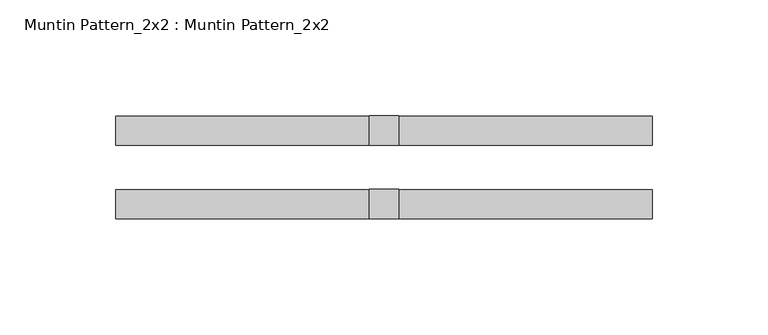
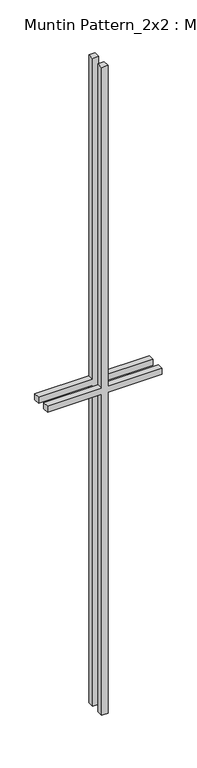
"""IFC4 building model written with IfcOpenShell, lengths in millimetres: proxy geometry, Muntin Pattern_2x2 : Muntin Pattern_2x2."""

from ifc_helpers import new_model, si_unit, frame, origin, place, context, project, spatial, polyline, outline, extrude, source, transform, mapped, element, save


def muntin_pattern_2x2_muntin_pattern_2x2_a2bda2b8(model_context):
    return source(origin(), model_context, "Body", "SweptSolid", [
        extrude(outline(polyline([(698.5, -6.35), (698.5, -115.8875), (685.8, -115.8875), (685.8, -6.35), (0.0, -6.35), (0.0, 6.35), (685.8, 6.35), (685.8, 115.8875), (698.5, 115.8875), (698.5, 6.35), (1384.3, 6.35), (1384.3, -6.35), (698.5, -6.35)])), frame((0.0, 9.525, 0.0), z_axis=(0.0, 1.0, 0.0), x_axis=(0.0, 0.0, 1.0)), (0.0, 0.0, 1.0), 12.7),
        extrude(outline(polyline([(698.5, -6.35), (698.5, -115.8875), (685.8, -115.8875), (685.8, -6.35), (0.0, -6.35), (0.0, 6.35), (685.8, 6.35), (685.8, 115.8875), (698.5, 115.8875), (698.5, 6.35), (1384.3, 6.35), (1384.3, -6.35), (698.5, -6.35)])), frame((0.0, -22.225, 0.0), z_axis=(0.0, 1.0, 0.0), x_axis=(0.0, 0.0, 1.0)), (0.0, 0.0, 1.0), 12.7),
    ])


if __name__ == "__main__":
    model = new_model("IFC4")
    model_context = context("Model", 3, world=origin())
    ifc_project = project(units=[si_unit("LENGTHUNIT", "METRE", prefix="MILLI")], contexts=[model_context])
    site = spatial("IfcSite", under=ifc_project)
    building = spatial("IfcBuilding", under=site)
    placement = place(None, origin())
    muntin_pattern_2x2_muntin_pattern_2x2_shape = muntin_pattern_2x2_muntin_pattern_2x2_a2bda2b8(model_context)
    element("IfcBuildingElementProxy", 1, Name="Muntin Pattern_2x2 : Muntin Pattern_2x2", ObjectType="Muntin Pattern_2x2 : Muntin Pattern_2x2", at=placement, inside=building, context=model_context, shape_type="MappedRepresentation", body=[
        mapped(muntin_pattern_2x2_muntin_pattern_2x2_shape, transform((0.0, 0.0, 0.0), x_axis=(1.0, 0.0, 0.0), y_axis=(0.0, 1.0, 0.0), z_axis=(0.0, 0.0, 1.0))),
    ])
    save(model, "model.ifc")

# Revit data of these elements
# Type "Muntin Pattern_2x2 : Muntin Pattern_2x2"
#   Width [instance default] = 4' - 0"
#   Thickness = 0' - 0 1/2"
#   Height [instance default] = 4' - 0"
#   Distance = 0' - 0 3/4"
#   Interior Material [instance default] = none
#   Exterior Material [instance default] = none
#   Default Elevation = 0
# Element 1 (IfcBuildingElementProxy, "Muntin Pattern_2x2 : Muntin Pattern_2x2")
#   Width = 0' - 9 1/8"
#   Height = 4' - 6 1/2"
#   Interior Material = Wood - Stained
#   Exterior Material = Clad - White
#   Materials on its faces: "Clad - White", "Wood - Stained"
# Materials
#   "Clad - White": class "Wood", colour RGB 242 242 238, transparency 0, Cost = 0
#   "Wood - Stained": class "Wood", colour RGB 224 178 126, transparency 0, Cost = 0
